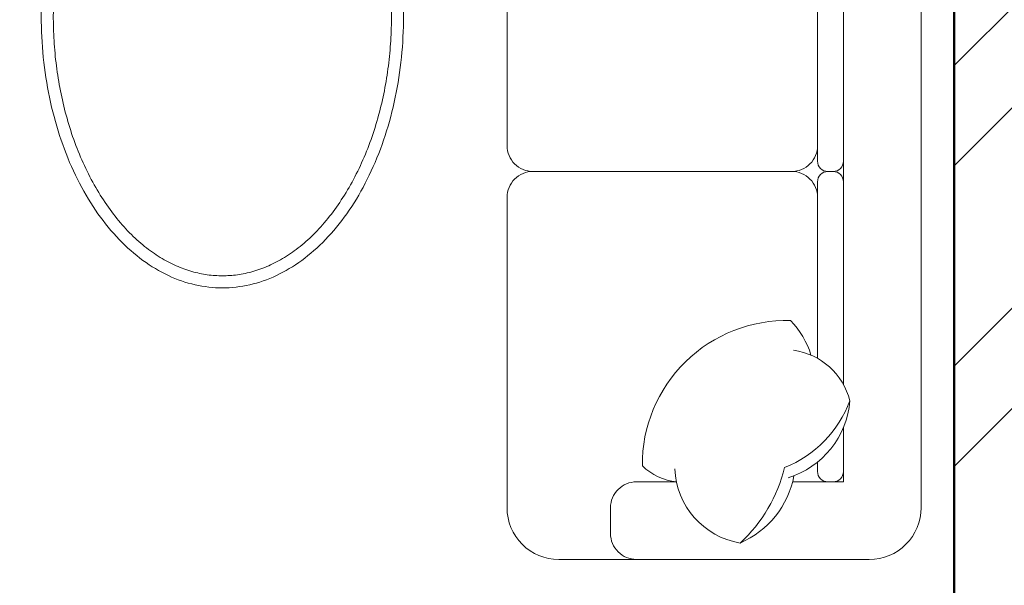
# Model space of a CAD drawing. Units: inches. Extents: x 963 to 2075, y 289 to 2657.
# Tile 74 of 98: x 1467 to 1511, y 2239 to 2265. Entities that reach past the tile are written whole.
import ezdxf

# ---------------------------------------------------------------- set-up
doc = ezdxf.new("R2010")
doc.units = ezdxf.units.IN
for name, color, linetype, lineweight in [('A-FURN', 8, 'Continuous', 18), ('A-WALL', 7, 'Continuous', 50), ('A-WALL-PATT', 8, 'Continuous', 13)]:
    doc.layers.add(name, color=color, linetype=linetype, lineweight=lineweight)

# ---------------------------------------------------------------- blocks, each defined once
blk = doc.blocks.new('TABLE-OVAL')
at = {"ltscale": 0.03}
blk.add_polyline3d([(7.656, -0.197, 0), (7.809, -0.194, 0), (7.963, -0.188, 0), (8.116, -0.177, 0), (8.269, -0.162, 0), (8.422, -0.142, 0), (8.575, -0.118, 0), (8.727, -0.09, 0), (8.879, -0.057, 0), (9.031, -0.021, 0), (9.182, 0.021, 0), (9.332, 0.066, 0), (9.482, 0.116, 0), (9.632, 0.17, 0), (9.78, 0.228, 0), (9.928, 0.29, 0), (10.075, 0.357, 0), (10.221, 0.428, 0), (10.366, 0.503, 0), (10.51, 0.582, 0), (10.653, 0.665, 0), (10.796, 0.752, 0), (10.937, 0.843, 0), (11.076, 0.938, 0), (11.215, 1.037, 0), (11.352, 1.14, 0), (11.488, 1.247, 0), (11.623, 1.358, 0), (11.756, 1.472, 0), (11.888, 1.59, 0), (12.018, 1.712, 0), (12.147, 1.838, 0), (12.274, 1.967, 0), (12.399, 2.1, 0), (12.523, 2.237, 0), (12.645, 2.376, 0), (12.765, 2.52, 0), (12.883, 2.666, 0), (13, 2.817, 0), (13.114, 2.97, 0), (13.227, 3.126, 0), (13.337, 3.286, 0), (13.446, 3.449, 0), (13.552, 3.615, 0), (13.657, 3.784, 0), (13.759, 3.955, 0), (13.859, 4.13, 0), (13.957, 4.308, 0), (14.052, 4.488, 0), (14.145, 4.671, 0), (14.236, 4.856, 0), (14.325, 5.044, 0), (14.411, 5.235, 0), (14.495, 5.428, 0), (14.576, 5.623, 0), (14.655, 5.821, 0), (14.731, 6.021, 0), (14.805, 6.222, 0), (14.877, 6.426, 0), (14.945, 6.632, 0), (15.011, 6.84, 0), (15.075, 7.05, 0), (15.135, 7.261, 0), (15.193, 7.475, 0), (15.249, 7.689, 0), (15.301, 7.906, 0), (15.351, 8.123, 0), (15.399, 8.343, 0), (15.443, 8.563, 0), (15.485, 8.785, 0), (15.523, 9.007, 0), (15.559, 9.231, 0), (15.592, 9.456, 0), (15.623, 9.682, 0), (15.65, 9.908, 0), (15.675, 10.136, 0), (15.697, 10.364, 0), (15.715, 10.592, 0), (15.731, 10.821, 0), (15.744, 11.051, 0), (15.755, 11.28, 0), (15.762, 11.51, 0), (15.766, 11.741, 0), (15.768, 11.971, 0), (15.766, 12.201, 0), (15.762, 12.431, 0), (15.755, 12.661, 0), (15.744, 12.891, 0), (15.731, 13.12, 0), (15.715, 13.349, 0), (15.697, 13.578, 0), (15.675, 13.806, 0), (15.65, 14.033, 0), (15.623, 14.26, 0), (15.592, 14.486, 0), (15.559, 14.71, 0), (15.523, 14.934, 0), (15.485, 15.157, 0), (15.443, 15.379, 0), (15.399, 15.599, 0), (15.351, 15.818, 0), (15.301, 16.036, 0), (15.249, 16.252, 0), (15.193, 16.467, 0), (15.135, 16.68, 0), (15.075, 16.892, 0), (15.011, 17.101, 0), (14.945, 17.309, 0), (14.877, 17.515, 0), (14.805, 17.719, 0), (14.731, 17.921, 0), (14.655, 18.121, 0), (14.576, 18.318, 0), (14.495, 18.514, 0), (14.411, 18.707, 0), (14.325, 18.897, 0), (14.236, 19.085, 0), (14.145, 19.271, 0), (14.052, 19.454, 0), (13.957, 19.634, 0), (13.859, 19.811, 0), (13.759, 19.986, 0), (13.657, 20.158, 0), (13.552, 20.327, 0), (13.446, 20.493, 0), (13.337, 20.656, 0), (13.227, 20.815, 0), (13.114, 20.972, 0), (13, 21.125, 0), (12.883, 21.275, 0), (12.765, 21.422, 0), (12.645, 21.565, 0), (12.523, 21.705, 0), (12.399, 21.842, 0), (12.274, 21.974, 0), (12.147, 22.104, 0), (12.018, 22.229, 0), (11.888, 22.351, 0), (11.756, 22.47, 0), (11.623, 22.584, 0), (11.488, 22.695, 0), (11.352, 22.802, 0), (11.215, 22.905, 0), (11.076, 23.004, 0), (10.937, 23.099, 0), (10.796, 23.19, 0), (10.653, 23.277, 0), (10.51, 23.36, 0), (10.366, 23.439, 0), (10.221, 23.514, 0), (10.075, 23.585, 0), (9.928, 23.651, 0), (9.78, 23.714, 0), (9.632, 23.772, 0), (9.482, 23.826, 0), (9.332, 23.876, 0), (9.182, 23.921, 0), (9.031, 23.962, 0), (8.879, 23.999, 0), (8.727, 24.032, 0), (8.575, 24.06, 0), (8.422, 24.084, 0), (8.269, 24.103, 0), (8.116, 24.119, 0), (7.963, 24.13, 0), (7.809, 24.136, 0), (7.656, 24.138, 0), (7.502, 24.136, 0), (7.349, 24.13, 0), (7.196, 24.119, 0), (7.042, 24.103, 0), (6.89, 24.084, 0), (6.737, 24.06, 0), (6.585, 24.032, 0), (6.433, 23.999, 0), (6.281, 23.962, 0), (6.13, 23.921, 0), (5.979, 23.876, 0), (5.83, 23.826, 0), (5.68, 23.772, 0), (5.532, 23.714, 0), (5.384, 23.651, 0), (5.237, 23.585, 0), (5.091, 23.514, 0), (4.946, 23.439, 0), (4.802, 23.36, 0), (4.658, 23.277, 0), (4.516, 23.19, 0), (4.375, 23.099, 0), (4.236, 23.004, 0), (4.097, 22.905, 0), (3.96, 22.802, 0), (3.824, 22.695, 0), (3.689, 22.584, 0), (3.556, 22.47, 0), (3.424, 22.351, 0), (3.294, 22.229, 0), (3.165, 22.104, 0), (3.038, 21.974, 0), (2.913, 21.842, 0), (2.789, 21.705, 0), (2.667, 21.565, 0), (2.547, 21.422, 0), (2.429, 21.275, 0), (2.312, 21.125, 0), (2.198, 20.972, 0), (2.085, 20.815, 0), (1.975, 20.656, 0), (1.866, 20.493, 0), (1.76, 20.327, 0), (1.655, 20.158, 0), (1.553, 19.986, 0), (1.453, 19.811, 0), (1.355, 19.634, 0), (1.26, 19.454, 0), (1.166, 19.271, 0), (1.076, 19.085, 0), (0.987, 18.897, 0), (0.901, 18.707, 0), (0.817, 18.514, 0), (0.736, 18.318, 0), (0.657, 18.121, 0), (0.58, 17.921, 0), (0.507, 17.719, 0), (0.435, 17.515, 0), (0.367, 17.309, 0), (0.301, 17.101, 0), (0.237, 16.892, 0), (0.177, 16.68, 0), (0.118, 16.467, 0), (0.063, 16.252, 0), (0.01, 16.036, 0), (-0.039, 15.818, 0), (-0.087, 15.599, 0), (-0.131, 15.379, 0), (-0.173, 15.157, 0), (-0.211, 14.934, 0), (-0.247, 14.71, 0), (-0.281, 14.486, 0), (-0.311, 14.26, 0), (-0.338, 14.033, 0), (-0.363, 13.806, 0), (-0.385, 13.578, 0), (-0.403, 13.349, 0), (-0.419, 13.12, 0), (-0.432, 12.891, 0), (-0.443, 12.661, 0), (-0.45, 12.431, 0), (-0.454, 12.201, 0), (-0.456, 11.971, 0), (-0.454, 11.741, 0), (-0.45, 11.51, 0), (-0.443, 11.28, 0), (-0.432, 11.051, 0), (-0.419, 10.821, 0), (-0.403, 10.592, 0), (-0.385, 10.364, 0), (-0.363, 10.136, 0), (-0.338, 9.908, 0), (-0.311, 9.682, 0), (-0.281, 9.456, 0), (-0.247, 9.231, 0), (-0.211, 9.007, 0), (-0.173, 8.785, 0), (-0.131, 8.563, 0), (-0.087, 8.343, 0), (-0.039, 8.123, 0), (0.01, 7.906, 0), (0.063, 7.689, 0), (0.118, 7.475, 0), (0.177, 7.261, 0), (0.237, 7.05, 0), (0.301, 6.84, 0), (0.367, 6.632, 0), (0.435, 6.426, 0), (0.507, 6.222, 0), (0.58, 6.021, 0), (0.657, 5.821, 0), (0.736, 5.623, 0), (0.817, 5.428, 0), (0.901, 5.235, 0), (0.987, 5.044, 0), (1.076, 4.856, 0), (1.166, 4.671, 0), (1.26, 4.488, 0), (1.355, 4.308, 0), (1.453, 4.13, 0), (1.553, 3.955, 0), (1.655, 3.784, 0), (1.76, 3.615, 0), (1.866, 3.449, 0), (1.975, 3.286, 0), (2.085, 3.126, 0), (2.198, 2.97, 0), (2.312, 2.817, 0), (2.429, 2.666, 0), (2.547, 2.52, 0), (2.667, 2.376, 0), (2.789, 2.237, 0), (2.913, 2.1, 0), (3.038, 1.967, 0), (3.165, 1.838, 0), (3.294, 1.712, 0), (3.424, 1.59, 0), (3.556, 1.472, 0), (3.689, 1.358, 0), (3.824, 1.247, 0), (3.96, 1.14, 0), (4.097, 1.037, 0), (4.236, 0.938, 0), (4.375, 0.843, 0), (4.516, 0.752, 0), (4.658, 0.665, 0), (4.802, 0.582, 0), (4.946, 0.503, 0), (5.091, 0.428, 0), (5.237, 0.357, 0), (5.384, 0.29, 0), (5.532, 0.228, 0), (5.68, 0.17, 0), (5.83, 0.116, 0), (5.979, 0.066, 0), (6.13, 0.021, 0), (6.281, -0.021, 0), (6.433, -0.057, 0), (6.585, -0.09, 0), (6.737, -0.118, 0), (6.89, -0.142, 0), (7.042, -0.162, 0), (7.196, -0.177, 0), (7.349, -0.188, 0), (7.502, -0.194, 0), (7.656, -0.197, 0)], dxfattribs=at)
blk.add_polyline3d([(7.656, 0.344, 0), (7.739, 0.345, 0), (7.822, 0.347, 0), (7.906, 0.351, 0), (7.99, 0.356, 0), (8.074, 0.362, 0), (8.159, 0.37, 0), (8.244, 0.38, 0), (8.33, 0.391, 0), (8.415, 0.404, 0), (8.501, 0.418, 0), (8.588, 0.434, 0), (8.674, 0.451, 0), (8.761, 0.47, 0), (8.848, 0.491, 0), (8.935, 0.513, 0), (9.023, 0.538, 0), (9.11, 0.563, 0), (9.198, 0.591, 0), (9.286, 0.62, 0), (9.375, 0.651, 0), (9.463, 0.684, 0), (9.552, 0.719, 0), (9.64, 0.755, 0), (9.729, 0.794, 0), (9.818, 0.834, 0), (9.907, 0.876, 0), (9.995, 0.92, 0), (10.084, 0.966, 0), (10.173, 1.013, 0), (10.262, 1.063, 0), (10.35, 1.114, 0), (10.439, 1.167, 0), (10.527, 1.222, 0), (10.615, 1.279, 0), (10.703, 1.338, 0), (10.791, 1.398, 0), (10.878, 1.461, 0), (10.965, 1.525, 0), (11.052, 1.592, 0), (11.139, 1.66, 0), (11.225, 1.73, 0), (11.311, 1.802, 0), (11.396, 1.876, 0), (11.481, 1.952, 0), (11.565, 2.03, 0), (11.649, 2.109, 0), (11.733, 2.191, 0), (11.815, 2.275, 0), (11.898, 2.361, 0), (11.98, 2.448, 0), (12.061, 2.537, 0), (12.141, 2.629, 0), (12.221, 2.721, 0), (12.301, 2.816, 0), (12.379, 2.912, 0), (12.457, 3.01, 0), (12.535, 3.11, 0), (12.611, 3.211, 0), (12.687, 3.314, 0), (12.762, 3.418, 0), (12.836, 3.524, 0), (12.909, 3.632, 0), (12.982, 3.741, 0), (13.053, 3.851, 0), (13.124, 3.963, 0), (13.194, 4.076, 0), (13.262, 4.191, 0), (13.33, 4.307, 0), (13.397, 4.424, 0), (13.463, 4.543, 0), (13.528, 4.662, 0), (13.591, 4.783, 0), (13.654, 4.906, 0), (13.716, 5.029, 0), (13.776, 5.154, 0), (13.835, 5.279, 0), (13.893, 5.406, 0), (13.95, 5.534, 0), (14.006, 5.663, 0), (14.061, 5.792, 0), (14.114, 5.923, 0), (14.166, 6.055, 0), (14.217, 6.188, 0), (14.266, 6.321, 0), (14.314, 6.455, 0), (14.361, 6.589, 0), (14.406, 6.723, 0), (14.45, 6.858, 0), (14.493, 6.993, 0), (14.535, 7.129, 0), (14.575, 7.265, 0), (14.614, 7.401, 0), (14.652, 7.537, 0), (14.688, 7.674, 0), (14.724, 7.811, 0), (14.758, 7.948, 0), (14.791, 8.086, 0), (14.822, 8.223, 0), (14.852, 8.361, 0), (14.882, 8.5, 0), (14.909, 8.638, 0), (14.936, 8.777, 0), (14.961, 8.916, 0), (14.986, 9.055, 0), (15.009, 9.194, 0), (15.031, 9.334, 0), (15.051, 9.473, 0), (15.071, 9.613, 0), (15.089, 9.753, 0), (15.106, 9.893, 0), (15.122, 10.033, 0), (15.137, 10.174, 0), (15.151, 10.314, 0), (15.163, 10.455, 0), (15.175, 10.596, 0), (15.185, 10.736, 0), (15.194, 10.877, 0), (15.202, 11.018, 0), (15.209, 11.159, 0), (15.215, 11.3, 0), (15.219, 11.441, 0), (15.223, 11.583, 0), (15.225, 11.724, 0), (15.227, 11.865, 0), (15.227, 12.006, 0), (15.226, 12.147, 0), (15.224, 12.288, 0), (15.221, 12.43, 0), (15.217, 12.571, 0), (15.212, 12.712, 0), (15.205, 12.853, 0), (15.198, 12.994, 0), (15.19, 13.135, 0), (15.18, 13.276, 0), (15.169, 13.416, 0), (15.157, 13.557, 0), (15.144, 13.698, 0), (15.13, 13.838, 0), (15.114, 13.978, 0), (15.098, 14.119, 0), (15.08, 14.259, 0), (15.061, 14.399, 0), (15.041, 14.538, 0), (15.02, 14.678, 0), (14.997, 14.817, 0), (14.974, 14.956, 0), (14.949, 15.095, 0), (14.923, 15.234, 0), (14.896, 15.373, 0), (14.867, 15.511, 0), (14.837, 15.649, 0), (14.806, 15.787, 0), (14.774, 15.925, 0), (14.741, 16.062, 0), (14.706, 16.199, 0), (14.67, 16.336, 0), (14.633, 16.473, 0), (14.595, 16.609, 0), (14.555, 16.745, 0), (14.514, 16.881, 0), (14.472, 17.016, 0), (14.428, 17.151, 0), (14.384, 17.286, 0), (14.338, 17.42, 0), (14.29, 17.554, 0), (14.241, 17.687, 0), (14.191, 17.821, 0), (14.14, 17.953, 0), (14.087, 18.084, 0), (14.034, 18.214, 0), (13.978, 18.344, 0), (13.922, 18.472, 0), (13.865, 18.599, 0), (13.806, 18.725, 0), (13.746, 18.85, 0), (13.685, 18.974, 0), (13.623, 19.097, 0), (13.56, 19.219, 0), (13.495, 19.339, 0), (13.43, 19.458, 0), (13.364, 19.576, 0), (13.296, 19.693, 0), (13.228, 19.808, 0), (13.159, 19.922, 0), (13.089, 20.035, 0), (13.017, 20.146, 0), (12.945, 20.255, 0), (12.873, 20.364, 0), (12.799, 20.47, 0), (12.724, 20.576, 0), (12.649, 20.679, 0), (12.573, 20.781, 0), (12.496, 20.882, 0), (12.418, 20.981, 0), (12.34, 21.078, 0), (12.261, 21.173, 0), (12.182, 21.267, 0), (12.101, 21.359, 0), (12.02, 21.449, 0), (11.939, 21.537, 0), (11.857, 21.624, 0), (11.774, 21.709, 0), (11.691, 21.791, 0), (11.607, 21.872, 0), (11.523, 21.951, 0), (11.438, 22.028, 0), (11.353, 22.103, 0), (11.268, 22.176, 0), (11.182, 22.247, 0), (11.095, 22.316, 0), (11.009, 22.383, 0), (10.922, 22.449, 0), (10.835, 22.512, 0), (10.747, 22.574, 0), (10.659, 22.633, 0), (10.571, 22.691, 0), (10.483, 22.747, 0), (10.395, 22.801, 0), (10.306, 22.854, 0), (10.217, 22.904, 0), (10.129, 22.952, 0), (10.04, 22.999, 0), (9.951, 23.044, 0), (9.862, 23.087, 0), (9.773, 23.128, 0), (9.685, 23.167, 0), (9.596, 23.205, 0), (9.507, 23.24, 0), (9.419, 23.274, 0), (9.331, 23.306, 0), (9.242, 23.336, 0), (9.154, 23.365, 0), (9.067, 23.391, 0), (8.979, 23.416, 0), (8.892, 23.44, 0), (8.804, 23.461, 0), (8.718, 23.481, 0), (8.631, 23.499, 0), (8.544, 23.516, 0), (8.458, 23.531, 0), (8.373, 23.545, 0), (8.287, 23.557, 0), (8.202, 23.567, 0), (8.117, 23.576, 0), (8.032, 23.583, 0), (7.948, 23.589, 0), (7.864, 23.593, 0), (7.781, 23.596, 0), (7.697, 23.597, 0), (7.615, 23.597, 0), (7.531, 23.596, 0), (7.448, 23.593, 0), (7.364, 23.589, 0), (7.28, 23.583, 0), (7.195, 23.576, 0), (7.11, 23.567, 0), (7.025, 23.557, 0), (6.939, 23.545, 0), (6.854, 23.531, 0), (6.767, 23.516, 0), (6.681, 23.499, 0), (6.594, 23.481, 0), (6.507, 23.461, 0), (6.42, 23.44, 0), (6.333, 23.416, 0), (6.245, 23.391, 0), (6.158, 23.365, 0), (6.07, 23.336, 0), (5.981, 23.306, 0), (5.893, 23.274, 0), (5.805, 23.24, 0), (5.716, 23.205, 0), (5.627, 23.167, 0), (5.539, 23.128, 0), (5.45, 23.087, 0), (5.361, 23.044, 0), (5.272, 22.999, 0), (5.183, 22.952, 0), (5.095, 22.904, 0), (5.006, 22.854, 0), (4.917, 22.801, 0), (4.829, 22.747, 0), (4.741, 22.691, 0), (4.653, 22.633, 0), (4.565, 22.574, 0), (4.477, 22.512, 0), (4.39, 22.449, 0), (4.303, 22.383, 0), (4.216, 22.316, 0), (4.13, 22.247, 0), (4.044, 22.176, 0), (3.959, 22.103, 0), (3.874, 22.028, 0), (3.789, 21.951, 0), (3.705, 21.872, 0), (3.621, 21.791, 0), (3.538, 21.709, 0), (3.455, 21.624, 0), (3.373, 21.537, 0), (3.292, 21.449, 0), (3.211, 21.359, 0), (3.13, 21.267, 0), (3.051, 21.173, 0), (2.972, 21.078, 0), (2.893, 20.981, 0), (2.816, 20.882, 0), (2.739, 20.781, 0), (2.663, 20.679, 0), (2.588, 20.576, 0), (2.513, 20.47, 0), (2.439, 20.364, 0), (2.366, 20.255, 0), (2.294, 20.146, 0), (2.223, 20.035, 0), (2.153, 19.922, 0), (2.084, 19.808, 0), (2.016, 19.693, 0), (1.948, 19.576, 0), (1.882, 19.458, 0), (1.817, 19.339, 0), (1.752, 19.219, 0), (1.689, 19.097, 0), (1.627, 18.974, 0), (1.566, 18.85, 0), (1.506, 18.725, 0), (1.447, 18.599, 0), (1.39, 18.472, 0), (1.334, 18.344, 0), (1.278, 18.214, 0), (1.225, 18.084, 0), (1.172, 17.953, 0), (1.121, 17.821, 0), (1.071, 17.687, 0), (1.022, 17.554, 0), (0.974, 17.42, 0), (0.928, 17.286, 0), (0.884, 17.151, 0), (0.84, 17.016, 0), (0.798, 16.881, 0), (0.757, 16.745, 0), (0.717, 16.609, 0), (0.679, 16.473, 0), (0.642, 16.336, 0), (0.606, 16.199, 0), (0.571, 16.062, 0), (0.538, 15.925, 0), (0.505, 15.787, 0), (0.475, 15.649, 0), (0.445, 15.511, 0), (0.416, 15.373, 0), (0.389, 15.234, 0), (0.363, 15.095, 0), (0.338, 14.956, 0), (0.315, 14.817, 0), (0.292, 14.678, 0), (0.271, 14.538, 0), (0.251, 14.399, 0), (0.232, 14.259, 0), (0.214, 14.119, 0), (0.198, 13.978, 0), (0.182, 13.838, 0), (0.168, 13.698, 0), (0.155, 13.557, 0), (0.143, 13.416, 0), (0.132, 13.276, 0), (0.122, 13.135, 0), (0.114, 12.994, 0), (0.106, 12.853, 0), (0.1, 12.712, 0), (0.095, 12.571, 0), (0.091, 12.43, 0), (0.088, 12.288, 0), (0.086, 12.147, 0), (0.085, 12.006, 0), (0.085, 11.865, 0), (0.087, 11.724, 0), (0.089, 11.583, 0), (0.093, 11.441, 0), (0.097, 11.3, 0), (0.103, 11.159, 0), (0.11, 11.018, 0), (0.118, 10.877, 0), (0.127, 10.736, 0), (0.137, 10.596, 0), (0.149, 10.455, 0), (0.161, 10.314, 0), (0.175, 10.174, 0), (0.19, 10.033, 0), (0.206, 9.893, 0), (0.223, 9.753, 0), (0.241, 9.613, 0), (0.261, 9.473, 0), (0.281, 9.334, 0), (0.303, 9.194, 0), (0.326, 9.055, 0), (0.35, 8.916, 0), (0.376, 8.777, 0), (0.403, 8.638, 0), (0.43, 8.5, 0), (0.46, 8.361, 0), (0.49, 8.223, 0), (0.521, 8.086, 0), (0.554, 7.948, 0), (0.588, 7.811, 0), (0.623, 7.674, 0), (0.66, 7.537, 0), (0.698, 7.401, 0), (0.737, 7.265, 0), (0.777, 7.129, 0), (0.819, 6.993, 0), (0.862, 6.858, 0), (0.906, 6.723, 0), (0.951, 6.589, 0), (0.998, 6.455, 0), (1.046, 6.321, 0), (1.095, 6.188, 0), (1.146, 6.055, 0), (1.198, 5.923, 0), (1.251, 5.792, 0), (1.306, 5.663, 0), (1.362, 5.534, 0), (1.418, 5.406, 0), (1.477, 5.279, 0), (1.536, 5.154, 0), (1.596, 5.029, 0), (1.658, 4.906, 0), (1.721, 4.783, 0), (1.784, 4.662, 0), (1.849, 4.543, 0), (1.915, 4.424, 0), (1.982, 4.307, 0), (2.05, 4.191, 0), (2.118, 4.076, 0), (2.188, 3.963, 0), (2.259, 3.851, 0), (2.33, 3.741, 0), (2.403, 3.632, 0), (2.476, 3.524, 0), (2.55, 3.418, 0), (2.625, 3.314, 0), (2.701, 3.211, 0), (2.777, 3.11, 0), (2.855, 3.01, 0), (2.933, 2.912, 0), (3.011, 2.816, 0), (3.09, 2.721, 0), (3.17, 2.629, 0), (3.251, 2.537, 0), (3.332, 2.448, 0), (3.414, 2.361, 0), (3.497, 2.275, 0), (3.579, 2.191, 0), (3.663, 2.109, 0), (3.747, 2.03, 0), (3.831, 1.952, 0), (3.916, 1.876, 0), (4.001, 1.802, 0), (4.087, 1.73, 0), (4.173, 1.66, 0), (4.26, 1.592, 0), (4.347, 1.525, 0), (4.434, 1.461, 0), (4.521, 1.398, 0), (4.609, 1.338, 0), (4.697, 1.279, 0), (4.785, 1.222, 0), (4.873, 1.167, 0), (4.962, 1.114, 0), (5.05, 1.063, 0), (5.139, 1.013, 0), (5.228, 0.966, 0), (5.316, 0.92, 0), (5.405, 0.876, 0), (5.494, 0.834, 0), (5.583, 0.794, 0), (5.672, 0.755, 0), (5.76, 0.719, 0), (5.849, 0.684, 0), (5.937, 0.651, 0), (6.026, 0.62, 0), (6.114, 0.591, 0), (6.201, 0.563, 0), (6.289, 0.538, 0), (6.377, 0.513, 0), (6.464, 0.491, 0), (6.551, 0.47, 0), (6.638, 0.451, 0), (6.724, 0.434, 0), (6.811, 0.418, 0), (6.897, 0.404, 0), (6.982, 0.391, 0), (7.068, 0.38, 0), (7.153, 0.37, 0), (7.237, 0.362, 0), (7.322, 0.356, 0), (7.406, 0.351, 0), (7.49, 0.347, 0), (7.573, 0.345, 0), (7.656, 0.344, 0)])

msp = doc.modelspace()

# ---------------------------------------------------------------- hatches: boundary and pattern name
at = {"layer": 'A-WALL-PATT'}
h = msp.add_hatch(dxfattribs=at)
h.set_pattern_fill('ANSI32', color=256)
h.paths.add_polyline_path([(1296.922, 2558.318), (1203.922, 2558.318), (1203.922, 2493.818), (1191.533, 2493.818), (1191.533, 2489.318), (1211.063, 2489.318), (1211.063, 2492.02), (1211.063, 2493.818), (1208.422, 2493.818), (1208.422, 2553.818), (1292.422, 2553.818), (1292.422, 2538.863), (1296.922, 2538.863)])
h.paths.add_polyline_path([(1442.422, 2558.318), (1349.422, 2558.318), (1349.422, 2538.943), (1353.922, 2538.943), (1353.922, 2553.818), (1437.922, 2553.818), (1437.922, 2493.818), (1434.542, 2493.818), (1434.542, 2489.318), (1448.311, 2489.318), (1448.311, 2491.568), (1448.311, 2493.818), (1442.422, 2493.818)])
h.paths.add_polyline_path([(1415.554, 2491.568), (1415.554, 2493.818), (1340.941, 2493.818), (1340.941, 2489.318), (1371.922, 2489.318), (1371.922, 2378.318), (1367.596, 2378.318), (1367.596, 2373.818), (1371.922, 2373.818), (1371.922, 2355.185), (1376.422, 2355.185), (1376.422, 2489.318), (1415.554, 2489.318)])
h.paths.add_polyline_path([(1304.941, 2491.568), (1304.941, 2493.818), (1296.922, 2493.818), (1296.922, 2514.863), (1292.422, 2514.863), (1292.422, 2493.818), (1232.808, 2493.818), (1232.808, 2489.318), (1256.422, 2489.318), (1256.422, 2327.318), (1253.714, 2327.318), (1253.714, 2322.818), (1328.422, 2322.818), (1328.422, 2331.147), (1323.922, 2331.147), (1323.922, 2327.318), (1260.922, 2327.318), (1260.922, 2373.818), (1323.922, 2373.818), (1323.922, 2357.812), (1328.422, 2357.812), (1328.422, 2373.818), (1346.007, 2373.818), (1346.007, 2376.068), (1346.007, 2378.318), (1260.922, 2378.318), (1260.922, 2489.318), (1304.941, 2489.318)])
h.paths.add_polyline_path([(1226.654, 2327.318), (1124.422, 2327.318), (1124.422, 2347.447), (1119.922, 2347.447), (1119.922, 2322.818), (1163.422, 2322.818), (1163.422, 2305.435), (1165.672, 2305.435), (1167.922, 2305.435), (1167.922, 2322.818), (1226.654, 2322.818), (1226.654, 2325.068)])
h.paths.add_polyline_path([(1095.922, 2489.318), (1124.422, 2489.318), (1131.533, 2489.318), (1131.533, 2491.568), (1131.533, 2493.818), (1119.922, 2493.818), (1091.422, 2493.818), (1091.422, 2417.318), (1095.922, 2417.318), (1119.922, 2417.318), (1119.922, 2407.447), (1124.422, 2407.447), (1124.422, 2421.818), (1095.922, 2421.818)])
h.paths.add_polyline_path([(1512.922, 2558.318), (1508.422, 2558.318), (1508.422, 2493.818), (1503.401, 2493.818), (1503.401, 2489.318), (1508.422, 2489.318), (1508.422, 2327.318), (1376.422, 2327.318), (1376.422, 2330.273), (1371.922, 2330.273), (1371.922, 2298.744), (1376.422, 2298.744), (1376.422, 2322.818), (1508.422, 2322.818), (1508.422, 2165.318), (1504.255, 2165.318), (1504.255, 2160.818), (1508.422, 2160.818), (1508.422, 2108.318), (1512.922, 2108.318), (1512.922, 2160.818), (1516.182, 2160.818), (1516.182, 2163.068), (1516.182, 2165.318), (1512.922, 2165.318), (1512.922, 2322.818), (1644.922, 2322.818), (1644.922, 2298.744), (1649.422, 2298.744), (1649.422, 2322.818), (1649.422, 2330.944), (1647.172, 2330.944), (1644.922, 2330.944), (1644.922, 2327.318), (1512.922, 2327.318), (1512.922, 2489.318), (1516.759, 2489.318), (1516.759, 2491.568), (1516.759, 2493.818), (1512.922, 2493.818)])
h.paths.add_polyline_path([(1671.922, 2558.318), (1578.922, 2558.318), (1578.922, 2493.818), (1573.526, 2493.818), (1573.526, 2489.318), (1586.537, 2489.318), (1586.537, 2491.568), (1586.537, 2493.818), (1583.422, 2493.818), (1583.422, 2553.818), (1667.422, 2553.818), (1667.422, 2541.109), (1671.922, 2541.109)])
h.paths.add_polyline_path([(1681.257, 2493.818), (1671.922, 2493.818), (1671.922, 2517.109), (1667.422, 2517.109), (1667.422, 2493.818), (1610.218, 2493.818), (1610.218, 2489.318), (1644.922, 2489.318), (1644.922, 2357.865), (1649.422, 2357.865), (1649.422, 2373.818), (1652.203, 2373.818), (1652.203, 2375.827), (1652.203, 2378.318), (1649.422, 2378.318), (1649.422, 2489.318), (1681.257, 2489.318), (1681.257, 2491.568)])
h.paths.add_polyline_path([(1821.922, 2558.318), (1728.922, 2558.318), (1728.922, 2541), (1733.422, 2541), (1733.422, 2553.818), (1817.422, 2553.818), (1817.422, 2493.818), (1813.507, 2493.818), (1813.507, 2489.318), (1830.078, 2489.318), (1830.078, 2491.568), (1830.078, 2493.818), (1821.922, 2493.818)])
h.paths.add_polyline_path([(1794.244, 2493.818), (1717.257, 2493.818), (1717.257, 2489.318), (1760.422, 2489.318), (1760.422, 2378.318), (1674.401, 2378.318), (1674.401, 2373.818), (1692.922, 2373.818), (1692.922, 2356.954), (1697.422, 2356.954), (1697.422, 2373.818), (1760.422, 2373.818), (1760.422, 2327.318), (1697.422, 2327.318), (1697.422, 2333.341), (1692.922, 2333.341), (1692.922, 2322.818), (1768.037, 2322.818), (1768.037, 2325.068), (1768.037, 2327.318), (1764.922, 2327.318), (1764.922, 2489.318), (1794.244, 2489.318)])
h.paths.add_polyline_path([(1733.422, 2517), (1728.922, 2517), (1728.922, 2493.818), (1733.422, 2493.818)], flags=17)
h.paths.add_polyline_path([(1929.922, 2493.818), (1890.078, 2493.818), (1890.078, 2489.318), (1896.922, 2489.318), (1925.422, 2489.318), (1925.422, 2421.818), (1896.922, 2421.818), (1896.922, 2408.318), (1901.422, 2408.318), (1901.422, 2417.318), (1925.422, 2417.318), (1929.922, 2417.318)])
h.paths.add_polyline_path([(1901.422, 2348.318), (1896.922, 2348.318), (1896.922, 2327.318), (1800.423, 2327.318), (1800.423, 2322.818), (1853.422, 2322.818), (1853.422, 2309.453), (1857.922, 2309.453), (1857.922, 2322.818), (1901.422, 2322.818)])
h.paths.add_polyline_path([(1857.922, 2249.453), (1853.422, 2249.453), (1853.422, 2214.818), (1686.309, 2214.818), (1686.309, 2210.318), (1853.422, 2210.318), (1853.422, 2202.134), (1857.922, 2202.134), (1857.922, 2210.318)])
h.paths.add_polyline_path([(1857.922, 2142.134), (1853.422, 2142.134), (1853.422, 2115.422), (1841.422, 2115.422), (1841.422, 2088.531), (1841.422, 2046.949), (1845.922, 2046.949), (1845.922, 2110.922), (1905.922, 2110.922), (1905.922, 2092.517), (1910.422, 2092.517), (1910.422, 2115.422), (1857.922, 2115.422)])
h.paths.add_polyline_path([(1532.436, 1482.342), (1573.456, 1482.342), (1573.456, 1501), (1532.436, 1501)], flags=9)
h.paths.add_polyline_path([(1438.658, 1486.302), (1479.678, 1486.302), (1479.678, 1504.96), (1438.658, 1504.96)], flags=9)
h.paths.add_polyline_path([(1411.215, 1365.308), (1659.139, 1365.308), (1659.139, 1402.401), (1411.215, 1402.401)], flags=9)
h.paths.add_polyline_path([(1185.671, 2296.298), (1248.16, 2296.298), (1248.16, 2314.955), (1185.671, 2314.955)], flags=9)
h.paths.add_polyline_path([(1177.31, 2187.35), (1216.15, 2187.35), (1216.15, 2206.007), (1177.31, 2206.007)], flags=9)
h.paths.add_polyline_path([(1295.101, 1602.083), (1328.26, 1602.083), (1328.26, 1620.741), (1295.101, 1620.741)], flags=9)
h.paths.add_polyline_path([(1525.126, 2005.99), (1558.39, 2005.99), (1558.39, 2024.648), (1525.126, 2024.648)], flags=9)
h.paths.add_polyline_path([(1459.606, 1977.125), (1472.195, 1977.125), (1472.195, 1987.429), (1459.606, 1987.429)], flags=9)
h.paths.add_polyline_path([(1467.815, 2053.676), (1480.018, 2053.676), (1480.018, 2063.979), (1467.815, 2063.979)], flags=9)
h.paths.add_polyline_path([(1555.184, 2119.02), (1584.563, 2119.02), (1584.563, 2137.678), (1555.184, 2137.678)], flags=25)
h.paths.add_polyline_path([(1405.389, 2115.291), (1444.478, 2115.291), (1444.478, 2133.948), (1405.389, 2133.948)], flags=25)
h.paths.add_polyline_path([(1698.482, 2004.259), (1727.695, 2004.259), (1727.695, 2022.916), (1698.482, 2022.916)], flags=9)
h.paths.add_polyline_path([(1612.158, 1972.855), (1629.016, 1972.855), (1629.016, 1983.159), (1612.158, 1983.159)], flags=9)
h.paths.add_polyline_path([(1608.289, 2060.036), (1625.147, 2060.036), (1625.147, 2070.34), (1608.289, 2070.34)], flags=9)
h.paths.add_polyline_path([(1527.954, 1684.402), (1566.795, 1684.402), (1566.795, 1703.06), (1527.954, 1703.06)], flags=9)
h.paths.add_polyline_path([(1422.792, 1683.59), (1461.633, 1683.59), (1461.633, 1702.247), (1422.792, 1702.247)], flags=9)
h.paths.add_polyline_path([(1531.262, 1732.459), (1574.015, 1732.459), (1574.015, 1751.116), (1531.262, 1751.116)], flags=9)
h.paths.add_polyline_path([(1402.872, 1732.845), (1439.799, 1732.845), (1439.799, 1751.502), (1402.872, 1751.502)], flags=9)
h.paths.add_polyline_path([(1243.122, 1923.132), (1281.962, 1923.132), (1281.962, 1941.79), (1243.122, 1941.79)], flags=9)
h.paths.add_polyline_path([(1181.752, 1792.268), (1244.241, 1792.268), (1244.241, 1810.926), (1181.752, 1810.926)], flags=9)
h.paths.add_polyline_path([(1265.822, 1670.3), (1316.071, 1670.3), (1316.071, 1688.957), (1265.822, 1688.957)], flags=9)
h.paths.add_polyline_path([(1140.263, 1676.054), (1179.104, 1676.054), (1179.104, 1694.711), (1140.263, 1694.711)], flags=9)
h.paths.add_polyline_path([(1107.49, 1490.889), (1143.374, 1490.889), (1143.374, 1509.546), (1107.49, 1509.546)], flags=9)
h.paths.add_polyline_path([(1217.584, 1483.899), (1246.741, 1483.899), (1246.741, 1502.556), (1217.584, 1502.556)], flags=9)
h.paths.add_polyline_path([(1389.21, 1486.919), (1418.367, 1486.919), (1418.367, 1505.576), (1389.21, 1505.576)], flags=9)
h.paths.add_polyline_path([(1672.208, 1602.083), (1705.366, 1602.083), (1705.366, 1620.741), (1672.208, 1620.741)], flags=9)
h.paths.add_polyline_path([(1752.082, 1522.638), (1781.24, 1522.638), (1781.24, 1541.295), (1752.082, 1541.295)], flags=9)
h.paths.add_polyline_path([(1848.275, 1491.26), (1884.158, 1491.26), (1884.158, 1509.918), (1848.275, 1509.918)], flags=9)
h.paths.add_polyline_path([(1822.47, 1685.62), (1861.31, 1685.62), (1861.31, 1704.278), (1822.47, 1704.278)], flags=9)
h.paths.add_polyline_path([(1713.195, 1672.232), (1763.444, 1672.232), (1763.444, 1690.889), (1713.195, 1690.889)], flags=9)
h.paths.add_polyline_path([(1736.619, 1790.578), (1799.109, 1790.578), (1799.109, 1809.235), (1736.619, 1809.235)], flags=9)
h.paths.add_polyline_path([(1691.491, 1916.355), (1730.332, 1916.355), (1730.332, 1935.013), (1691.491, 1935.013)], flags=9)
h.paths.add_polyline_path([(1764.872, 1973.922), (1794.306, 1973.922), (1794.306, 1992.58), (1764.872, 1992.58)], flags=9)
h.paths.add_polyline_path([(1767.854, 2034.017), (1797.288, 2034.017), (1797.288, 2052.674), (1767.854, 2052.674)], flags=9)
h.paths.add_polyline_path([(1851.593, 2060.331), (1880.751, 2060.331), (1880.751, 2078.989), (1851.593, 2078.989)], flags=25)
h.paths.add_polyline_path([(1688.491, 2086.874), (1727.332, 2086.874), (1727.332, 2105.531), (1688.491, 2105.531)], flags=9)
h.paths.add_polyline_path([(1537.743, 2293.581), (1580.495, 2293.581), (1580.495, 2312.239), (1537.743, 2312.239)], flags=25)
h.paths.add_polyline_path([(1425.587, 2296.109), (1468.34, 2296.109), (1468.34, 2314.766), (1425.587, 2314.766)], flags=25)
h.paths.add_polyline_path([(1278.518, 2004.184), (1307.72, 2004.184), (1307.72, 2022.841), (1278.518, 2022.841)], flags=9)
h.paths.add_polyline_path([(1193.282, 1973.635), (1222.715, 1973.635), (1222.715, 1992.292), (1193.282, 1992.292)], flags=9)
h.paths.add_polyline_path([(1192.411, 2040.577), (1221.845, 2040.577), (1221.845, 2059.234), (1192.411, 2059.234)], flags=9)
h.paths.add_polyline_path([(1130.603, 1951.393), (1159.76, 1951.393), (1159.76, 1970.05), (1130.603, 1970.05)], flags=9)
h.paths.add_polyline_path([(1132.827, 2052.494), (1161.984, 2052.494), (1161.984, 2071.151), (1132.827, 2071.151)], flags=9)
h.paths.add_polyline_path([(1265.128, 2334.619), (1315.377, 2334.619), (1315.377, 2353.277), (1265.128, 2353.277)], flags=25)
h.paths.add_polyline_path([(1136.741, 2330.785), (1175.582, 2330.785), (1175.582, 2349.443), (1136.741, 2349.443)], flags=9)
h.paths.add_polyline_path([(1287.422, 2417.204), (1320.58, 2417.204), (1320.58, 2435.861), (1287.422, 2435.861)], flags=25)
h.paths.add_polyline_path([(1430.988, 2329.159), (1469.828, 2329.159), (1469.828, 2347.816), (1430.988, 2347.816)], flags=25)
h.paths.add_polyline_path([(1525.424, 2329.213), (1564.264, 2329.213), (1564.264, 2347.87), (1525.424, 2347.87)], flags=25)
h.paths.add_polyline_path([(1684.525, 2382.799), (1717.683, 2382.799), (1717.683, 2401.457), (1684.525, 2401.457)], flags=25)
h.paths.add_polyline_path([(1704.805, 2340.293), (1755.054, 2340.293), (1755.054, 2358.95), (1704.805, 2358.95)], flags=25)
h.paths.add_polyline_path([(1694.113, 2287.757), (1756.602, 2287.757), (1756.602, 2306.414), (1694.113, 2306.414)], flags=9)
h.paths.add_polyline_path([(1815.778, 2329.861), (1854.618, 2329.861), (1854.618, 2348.518), (1815.778, 2348.518)], flags=9)
h.paths.add_polyline_path([(1842.873, 2514.256), (1878.756, 2514.256), (1878.756, 2532.914), (1842.873, 2532.914)], flags=9)
h.paths.add_polyline_path([(1769.513, 2531.447), (1798.671, 2531.447), (1798.671, 2550.104), (1769.513, 2550.104)], flags=25)
h.paths.add_polyline_path([(1594.772, 2518.468), (1623.93, 2518.468), (1623.93, 2537.125), (1594.772, 2537.125)], flags=25)
h.paths.add_polyline_path([(1520.723, 2516.185), (1556.606, 2516.185), (1556.606, 2534.842), (1520.723, 2534.842)], flags=25)
h.paths.add_polyline_path([(1464.456, 2516.694), (1500.34, 2516.694), (1500.34, 2535.351), (1464.456, 2535.351)], flags=25)
h.paths.add_polyline_path([(1365.696, 2528.97), (1394.854, 2528.97), (1394.854, 2547.627), (1365.696, 2547.627)], flags=25)
h.paths.add_polyline_path([(1222.838, 2516.231), (1251.995, 2516.231), (1251.995, 2534.889), (1222.838, 2534.889)], flags=25)
h.paths.add_polyline_path([(1104.545, 2509.6), (1140.429, 2509.6), (1140.429, 2528.257), (1104.545, 2528.257)], flags=9)

# ---------------------------------------------------------------- linework, layer by layer
at = {"layer": 'A-FURN', "ltscale": 0.03}
msp.add_lwpolyline([(1490.72, 2240.636, -0.414214), (1488.403, 2242.954), (1488.403, 2256.859, -0.414214), (1489.562, 2258.018, -0.414214), (1488.403, 2259.177), (1488.403, 2270.765, -0.414214), (1489.562, 2271.924, -0.414214), (1488.403, 2273.082), (1488.403, 2286.988, -0.414214), (1490.72, 2289.306), (1504.626, 2289.306, -0.414214), (1506.944, 2286.988), (1506.944, 2242.954, -0.414214), (1504.626, 2240.636)], format="xyb", close=True, dxfattribs=at)
at = {"layer": 'A-FURN'}
for points in [[(1503.467, 2248.478), (1503.467, 2275.221)], [(1501.19, 2244.112), (1503.467, 2244.112), (1503.467, 2246.55)]]:
    msp.add_lwpolyline(points, dxfattribs=at)
msp.add_lwpolyline([(1503.467, 2271.46), (1503.467, 2258.482, -0.414214), (1503.004, 2258.018), (1502.772, 2258.018, -0.414214), (1502.308, 2258.482), (1502.308, 2271.46, -0.414214), (1502.772, 2271.924), (1503.004, 2271.924, -0.414214)], format="xyb", close=True, dxfattribs=at)
for points in [[(1502.308, 2259.177, -0.414214), (1501.15, 2258.018)], [(1502.308, 2256.859, 0.414214), (1501.15, 2258.018), (1489.562, 2258.018, 0.414214)], [(1503.467, 2248.478), (1503.467, 2257.554, 0.414214), (1503.004, 2258.018), (1502.772, 2258.018, 0.414214), (1502.308, 2257.554), (1502.308, 2249.645, 0.414214)], [(1495.993, 2244.11, -0.165541), (1494.462, 2244.827, -0.425989), (1501.1, 2251.335, -0.121523), (1502.015, 2249.79, 7.115464)], [(1500.993, 2244.292, 0.306663), (1503.755, 2247.749, 0.30633), (1501.233, 2250.007, -0.872847)], [(1498.843, 2241.373, 0.14773), (1500.835, 2244.76, 0.213343), (1503.755, 2247.749, 0.178662)], [(1503.467, 2244.576), (1503.467, 2246.55, 0.414214)], [(1502.308, 2244.997), (1502.308, 2244.576, 0.414214), (1502.772, 2244.112), (1503.004, 2244.112, 0.414214), (1503.467, 2244.576)], [(1495.922, 2244.694, 0.356772), (1498.843, 2241.373, 0.249542), (1501.25, 2244.382, -9.61688)], [(1494.197, 2240.636, -0.414214), (1493.038, 2241.795), (1493.038, 2242.954, -0.414214), (1494.197, 2244.112), (1495.992, 2244.112)]]:
    msp.add_lwpolyline(points, format="xyb", dxfattribs=at)
at = {"layer": 'A-WALL'}
msp.add_line((1508.422, 2322.818), (1508.422, 2165.318), dxfattribs=at)

# ---------------------------------------------------------------- block references
at = {"layer": 'A-FURN'}
msp.add_blockref('TABLE-OVAL', (1468, 2253), dxfattribs=at)

doc.saveas('drawing.dxf')
